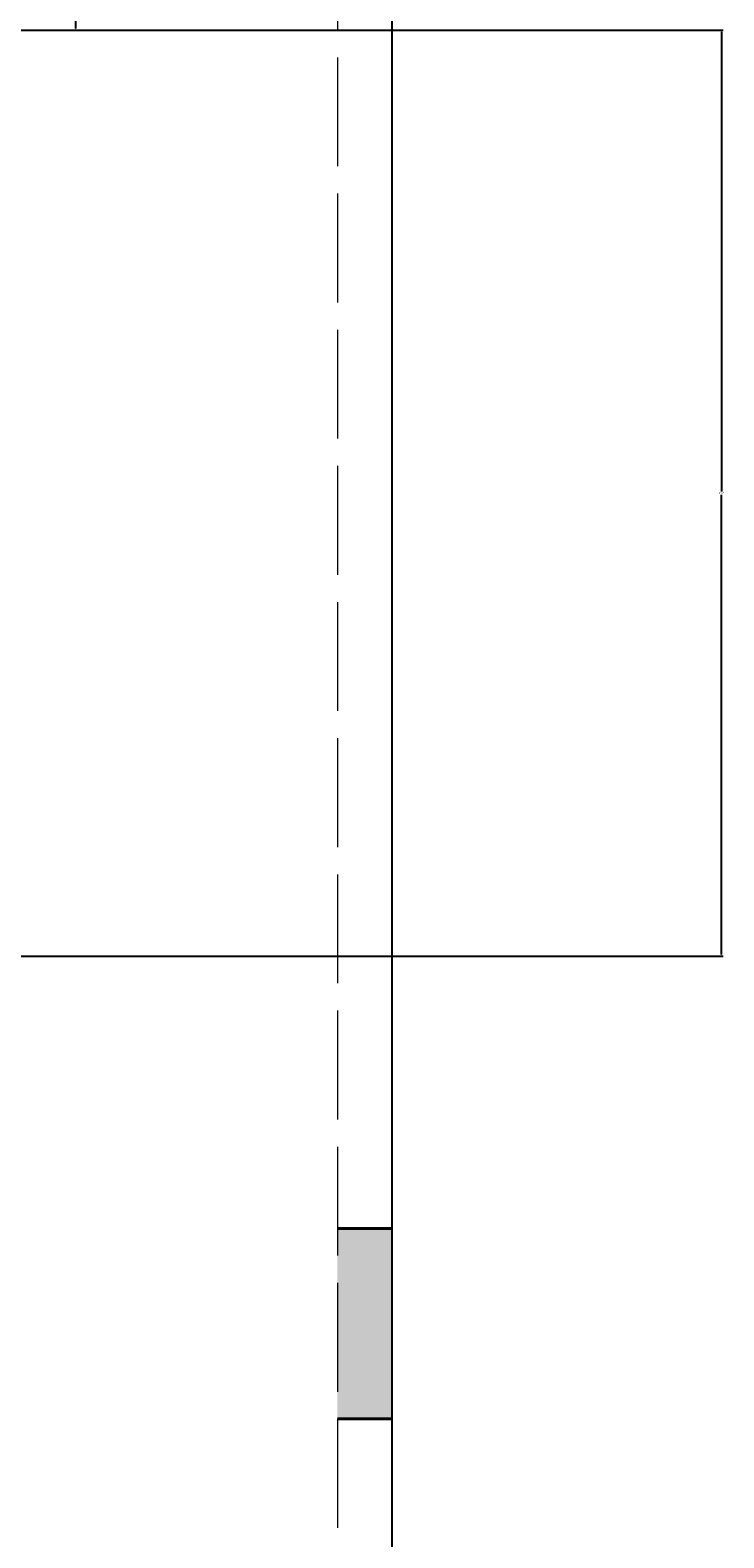
# Model space of a CAD drawing. Units: inches. Extents: x -36 to 401, y -686 to 73.
# Tile 10 of 15: x 325 to 401, y -485 to -319. Entities that reach past the tile are written whole.
import ezdxf

# ---------------------------------------------------------------- set-up
doc = ezdxf.new("R2010")
doc.units = ezdxf.units.IN
doc.header["$MEASUREMENT"] = 0
doc.linetypes.add('ACAD_ISO02W100', pattern=[15, 12, -3])
for name, color, linetype, lineweight in [('A-ANNO-DIMS', 2, 'Continuous', 18), ('A-COLS', 7, 'Continuous', 40), ('A-COLS-PATT', 22, 'Continuous', 13), ('A-FLOR-OVHD', 8, 'ACAD_ISO02W100', 18), ('C-PROP', 7, 'Continuous', 25)]:
    doc.layers.add(name, color=color, linetype=linetype, lineweight=lineweight)
doc.styles.get("Standard").update_dxf_attribs({"font": 'arial.ttf'})
doc.dimstyles.get("Standard").update_dxf_attribs({"dimtxt": 0.18, "dimasz": 0.18, "dimexe": 0.18, "dimexo": 0.0625, "dimgap": 0.09, "dimtad": 0, "dimtih": 1, "dimtoh": 1, "dimdec": 0, "dimzin": 0, "dimdsep": 46, "dimlunit": 3, "dimtxsty": 'Standard', "dimcen": 0.09, "dimadec": 0, "dimazin": 0, "dimtfac": 1, "dimtdec": 0, "dimtofl": 0, "dimtmove": 0, "dimatfit": 3, "dimfxl": 1, "dimtolj": 1, "dimtzin": 0, "dimarcsym": 0})

# ---------------------------------------------------------------- blocks, each defined once
blk = doc.blocks.new('*D45')
at = {"layer": 'A-ANNO-DIMS', "color": 0, "lineweight": -2, "transparency": 16777216}
for p, q in [((322.75, -271.21), (330.07, -271.21)), ((329.89, -271.39), (329.89, -295.03)), ((329.89, -319.03), (329.89, -295.39)), ((322.75, -319.21), (330.07, -319.21))]:
    blk.add_line(p, q, dxfattribs=at)
at = {"layer": 'A-ANNO-DIMS', "color": 0, "transparency": 16777216}
for points in [[(329.86, -271.39), (329.92, -271.39), (329.89, -271.21)], [(329.86, -319.03), (329.92, -319.03), (329.89, -319.21)]]:
    blk.add_solid(points, dxfattribs=at)
at = {"layer": 'Defpoints', "color": 0, "transparency": 16777216}
for p in [(322.69, -271.21), (329.89, -271.21), (322.69, -319.21)]:
    blk.add_point(p, dxfattribs=at)
at = {"layer": 'A-ANNO-DIMS', "color": 0, "transparency": 16777216, "insert": (329.89, -295.21), "char_height": 0.18, "attachment_point": 5}
blk.add_mtext('\\A1;DOOR PAIR 4\'-0" TYP.', dxfattribs=at)
blk = doc.blocks.new('*D72')
at = {"layer": 'A-ANNO-DIMS', "color": 0, "lineweight": -2, "transparency": 16777216}
for p, q in [((322.75, -319.21), (401.17, -319.21)), ((400.99, -319.39), (400.99, -370.03)), ((400.99, -421.03), (400.99, -370.39)), ((322.75, -421.21), (401.17, -421.21))]:
    blk.add_line(p, q, dxfattribs=at)
at = {"layer": 'A-ANNO-DIMS', "color": 0, "transparency": 16777216}
for points in [[(400.96, -319.39), (401.02, -319.39), (400.99, -319.21)], [(400.96, -421.03), (401.02, -421.03), (400.99, -421.21)]]:
    blk.add_solid(points, dxfattribs=at)
at = {"layer": 'Defpoints', "color": 0, "transparency": 16777216}
for p in [(322.69, -319.21), (322.69, -421.21), (400.99, -421.21)]:
    blk.add_point(p, dxfattribs=at)
at = {"layer": 'A-ANNO-DIMS', "color": 0, "transparency": 16777216, "insert": (400.99, -370.21), "char_height": 0.18, "attachment_point": 5}
blk.add_mtext('\\A1;8\'-6"', dxfattribs=at)

msp = doc.modelspace()

# ---------------------------------------------------------------- hatches: boundary and pattern name
at = {"layer": 'A-COLS-PATT'}
h = msp.add_hatch(color=256, dxfattribs=at)
h.dxf.hatch_style = 1
h.paths.add_polyline_path([(34.69, 7.79), (25.69, 7.79), (25.69, -13.21), (34.69, -13.21)])
h.paths.add_polyline_path([(172.69, -13.21), (177.19, -13.21), (181.69, -13.21), (181.69, 7.79), (172.69, 7.79)])
h.paths.add_polyline_path([(322.69, 7.79), (313.69, 7.79), (313.69, -13.21), (322.69, -13.21)])
h.paths.add_polyline_path([(322.69, -157.21), (313.69, -157.21), (313.69, -178.21), (322.69, -178.21)])
h.paths.add_polyline_path([(172.69, -178.21), (177.19, -178.21), (181.69, -178.21), (181.69, -157.21), (177.19, -157.21), (172.69, -157.21)])
h.paths.add_polyline_path([(25.69, -178.21), (34.69, -178.21), (34.69, -157.21), (25.69, -157.21)])
h.paths.add_polyline_path([(34.69, -325.21), (25.69, -325.21), (25.69, -346.21), (34.69, -346.21)])
h.paths.add_polyline_path([(181.69, -325.21), (177.19, -325.21), (172.69, -325.21), (172.69, -346.21), (177.19, -346.21), (181.69, -346.21)])
h.paths.add_polyline_path([(322.69, -325.21), (313.69, -325.21), (313.69, -346.21), (322.69, -346.21)])
h.paths.add_polyline_path([(364.69, -451.21), (358.69, -451.21), (358.69, -472.21), (364.69, -472.21)])
h.paths.add_polyline_path([(181.69, -451.21), (177.19, -451.21), (172.69, -451.21), (172.69, -472.21), (177.19, -472.21), (181.69, -472.21)])
h.paths.add_polyline_path([(25.69, -472.21), (34.69, -472.21), (34.69, -451.21), (25.69, -451.21)])

# ---------------------------------------------------------------- linework, layer by layer
at = {"layer": 'A-COLS'}
for p, q in [((358.69, -451.21), (364.69, -451.21)), ((358.69, -472.21), (364.69, -472.21))]:
    msp.add_line(p, q, dxfattribs=at)
at = {"layer": 'A-FLOR-OVHD'}
msp.add_line((358.69, 7.79), (358.69, -559.77), dxfattribs=at)
at = {"layer": 'C-PROP'}
msp.add_line((364.69, 31.79), (364.69, -649.21), dxfattribs=at)

# ---------------------------------------------------------------- dimensions: what is measured, and where the dimension line sits
at = {"layer": 'A-ANNO-DIMS'}
dim = msp.add_linear_dim(base=(329.89, -271.21), p1=(322.69, -319.21), p2=(322.69, -271.21), angle=90, text='DOOR PAIR <> TYP.', dimstyle='Standard', override={"dimdec": 1, "dimlfac": 1, "dimrnd": 0, "dimzin": 1, "dimdsep": 46, "dimlunit": 4, "dimfrac": 2}, dxfattribs=at)
dim.commit()
dim.dimension.update_dxf_attribs({"geometry": '*D45', "text_midpoint": (329.89, -295.21)})
dim = msp.add_linear_dim(base=(400.99, -421.21), p1=(322.69, -319.21), p2=(322.69, -421.21), angle=90, dimstyle='Standard', override={"dimdec": 1, "dimlfac": 1, "dimrnd": 0, "dimzin": 1, "dimdsep": 46, "dimlunit": 4, "dimfrac": 2}, dxfattribs=at)
dim.commit()
dim.dimension.update_dxf_attribs({"geometry": '*D72', "text_midpoint": (400.99, -370.21)})

doc.saveas('drawing.dxf')
